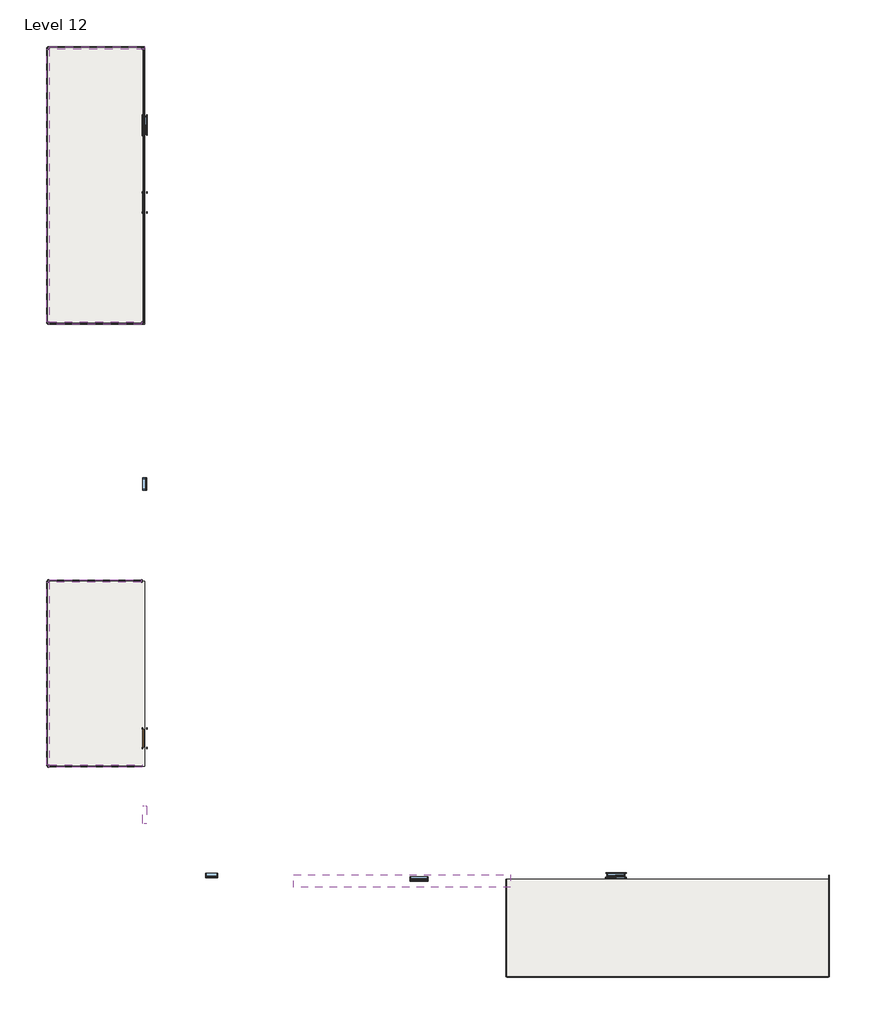
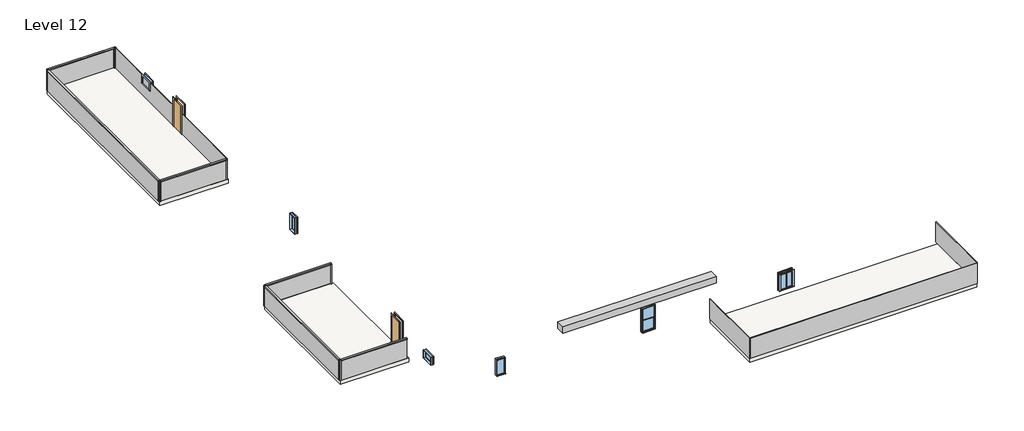
# One storey: 17 members, 10 plates, 6 windows, 3 slabs, 2 doors, 1 proxy.
"""IFC4 building model written with IfcOpenShell, lengths in millimetres."""

from ifc_helpers import new_model, si_unit, frame, origin, place, context, project, spatial, polyline, outline, extrude, transform, mapped, element, save
from components import generic_models_5_generic_models_5_6f0b94fe, door_54dd4da4, member_a0ba9e48, member_4491d118, member_6d14b308, member_9867d003, member_a33656d8, member_5f6c94d3, member_61d9bab4, system_panel_glazed_6303489a, system_panel_glazed_dbf8c7ac, system_panel_glazed_b7a52489, system_panel_glazed_1f759628, system_panel_glazed_82bc3a22, system_panel_glazed_e6d06af6, system_panel_glazed_929cc49f, system_panel_glazed_21f26c1a, system_panel_glazed_1fde7296, system_panel_glazed_b34c6f43, window_f274a882, window_80bd9af0, window_57c3ee1c, window_78885257, window_a4355bb3, window_54100e87

model = new_model("IFC4")

# Units and contexts
model_context = context("Model", 3, world=origin())
ifc_project = project(units=[si_unit("LENGTHUNIT", "METRE", prefix="MILLI")], contexts=[model_context])

# Site, building, storey
site = spatial("IfcSite", under=ifc_project)
building = spatial("IfcBuilding", under=site)
storey = spatial("IfcBuildingStorey", under=building, Name="Level 12", Elevation=19812.0)

# Proxy
placement = place(None, origin())
generic_models_5_generic_models_5_shape = generic_models_5_generic_models_5_6f0b94fe(model_context)
element("IfcBuildingElementProxy", 1, Name="Generic Models 5 : Generic Models 5", ObjectType="Generic Models 5 : Generic Models 5", at=placement, inside=storey, context=model_context, shape_type="MappedRepresentation", body=[
    mapped(generic_models_5_generic_models_5_shape, transform((508.0, 127.0, 0.0), x_axis=(1.0, 0.0, 0.0), y_axis=(0.0, 1.0, 0.0), z_axis=(0.0, 0.0, 1.0))),
])

# Doors
door_shape = door_54dd4da4(model_context)
element("IfcDoor", 2, ObjectType="Single-Flush : 36\" x 84\"", at=placement, inside=storey, context=model_context, shape_type="MappedRepresentation", body=[
    mapped(door_shape, transform((-15175.038074, 13037.8014639, 19812.0), x_axis=(0.0, 1.0, 0.0), y_axis=(-1.0, 0.0, 0.0), z_axis=(0.0, 0.0, 1.0))),
])
element("IfcDoor", 3, ObjectType="Single-Flush : 36\" x 84\"", at=placement, inside=storey, context=model_context, shape_type="MappedRepresentation", body=[
    mapped(door_shape, transform((-15175.038074, -13852.5915889, 19812.0), x_axis=(0.0, 1.0, 0.0), y_axis=(-1.0, 0.0, 0.0), z_axis=(0.0, 0.0, 1.0))),
])

# Members
member_shape = member_a0ba9e48(model_context)
element("IfcMember", 4, ObjectType="Rectangular Mullion : 2.5\" x 5\" rectangular", at=placement, inside=storey, context=model_context, shape_type="MappedRepresentation", body=[
    mapped(member_shape, transform((-15175.038074, 20810.2014639, 21336.0), x_axis=(0.0, 0.0, 1.0), y_axis=(0.0, -1.0, 0.0), z_axis=(1.0, 0.0, 0.0))),
])
member_2_shape = member_4491d118(model_context)
element("IfcMember", 5, ObjectType="Rectangular Mullion : 2.5\" x 5\" rectangular", at=placement, inside=storey, context=model_context, shape_type="MappedRepresentation", body=[
    mapped(member_2_shape, transform((-20051.838074, 20810.2014639, 19812.0), x_axis=(0.0, 1.0, 0.0), y_axis=(1.0, 0.0, 0.0), z_axis=(0.0, 0.0, -1.0))),
])
element("IfcMember", 6, ObjectType="Rectangular Mullion : 2.5\" x 5\" rectangular", at=placement, inside=storey, context=model_context, shape_type="MappedRepresentation", body=[
    mapped(member_2_shape, transform((-20051.838074, 6991.7543143, 19812.0), x_axis=(-1.0, 0.0, 0.0), y_axis=(0.0, 1.0, 0.0), z_axis=(0.0, 0.0, -1.0))),
])
element("IfcMember", 7, ObjectType="Rectangular Mullion : 2.5\" x 5\" rectangular", at=placement, inside=storey, context=model_context, shape_type="MappedRepresentation", body=[
    mapped(member_2_shape, transform((-15308.388074, -5966.8213044, 19812.0), x_axis=(1.0, 0.0, 0.0), y_axis=(0.0, -1.0, 0.0), z_axis=(0.0, 0.0, -1.0))),
])
element("IfcMember", 8, ObjectType="Rectangular Mullion : 2.5\" x 5\" rectangular", at=placement, inside=storey, context=model_context, shape_type="MappedRepresentation", body=[
    mapped(member_2_shape, transform((-20051.838074, -5966.8213044, 19812.0), x_axis=(0.0, 1.0, 0.0), y_axis=(1.0, 0.0, 0.0), z_axis=(0.0, 0.0, -1.0))),
])
element("IfcMember", 9, ObjectType="Rectangular Mullion : 2.5\" x 5\" rectangular", at=placement, inside=storey, context=model_context, shape_type="MappedRepresentation", body=[
    mapped(member_2_shape, transform((-20051.838074, -15250.5213044, 19812.0), x_axis=(-1.0, 0.0, 0.0), y_axis=(0.0, 1.0, 0.0), z_axis=(0.0, 0.0, -1.0))),
])
element("IfcMember", 10, ObjectType="Rectangular Mullion : 2.5\" x 5\" rectangular", at=placement, inside=storey, context=model_context, shape_type="MappedRepresentation", body=[
    mapped(member_2_shape, transform((-20051.838074, 20810.2014639, 21336.0), x_axis=(-1.0, 0.0, 0.0), y_axis=(0.0, -1.0, 0.0), z_axis=(0.0, 0.0, 1.0))),
])
element("IfcMember", 11, ObjectType="Rectangular Mullion : 2.5\" x 5\" rectangular", at=placement, inside=storey, context=model_context, shape_type="MappedRepresentation", body=[
    mapped(member_2_shape, transform((-20051.838074, 6991.7543143, 21336.0), x_axis=(0.0, -1.0, 0.0), y_axis=(1.0, 0.0, 0.0), z_axis=(0.0, 0.0, 1.0))),
])
element("IfcMember", 12, ObjectType="Rectangular Mullion : 2.5\" x 5\" rectangular", at=placement, inside=storey, context=model_context, shape_type="MappedRepresentation", body=[
    mapped(member_2_shape, transform((-15276.638074, 6991.7543143, 21336.0), x_axis=(1.0, 0.0, 0.0), y_axis=(0.0, 1.0, 0.0), z_axis=(0.0, 0.0, 1.0))),
])
element("IfcMember", 13, ObjectType="Rectangular Mullion : 2.5\" x 5\" rectangular", at=placement, inside=storey, context=model_context, shape_type="MappedRepresentation", body=[
    mapped(member_2_shape, transform((-20051.838074, -5966.8213044, 21336.0), x_axis=(-1.0, 0.0, 0.0), y_axis=(0.0, -1.0, 0.0), z_axis=(0.0, 0.0, 1.0))),
])
element("IfcMember", 14, ObjectType="Rectangular Mullion : 2.5\" x 5\" rectangular", at=placement, inside=storey, context=model_context, shape_type="MappedRepresentation", body=[
    mapped(member_2_shape, transform((-20051.838074, -15250.5213044, 21336.0), x_axis=(0.0, -1.0, 0.0), y_axis=(1.0, 0.0, 0.0), z_axis=(0.0, 0.0, 1.0))),
])
member_3_shape = member_6d14b308(model_context)
element("IfcMember", 15, ObjectType="Rectangular Mullion : 2.5\" x 5\" rectangular", at=placement, inside=storey, context=model_context, shape_type="MappedRepresentation", body=[
    mapped(member_3_shape, transform((-19988.338074, 6991.7543143, 21336.0), x_axis=(0.0, 0.0, 1.0), y_axis=(0.0, 1.0, 0.0), z_axis=(-1.0, 0.0, 0.0))),
])
element("IfcMember", 16, ObjectType="Rectangular Mullion : 2.5\" x 5\" rectangular", at=placement, inside=storey, context=model_context, shape_type="MappedRepresentation", body=[
    mapped(member_2_shape, transform((-15276.638074, 20810.2014639, 21336.0), x_axis=(0.0, 1.0, 0.0), y_axis=(-1.0, 0.0, 0.0), z_axis=(0.0, 0.0, 1.0))),
])
member_4_shape = member_9867d003(model_context)
element("IfcMember", 17, ObjectType="Rectangular Mullion : 2.5\" x 5\" rectangular", at=placement, inside=storey, context=model_context, shape_type="MappedRepresentation", body=[
    mapped(member_4_shape, transform((-20051.838074, 20746.7014639, 21336.0), x_axis=(0.0, 0.0, 1.0), y_axis=(1.0, 0.0, 0.0), z_axis=(0.0, 1.0, 0.0))),
])
member_5_shape = member_a33656d8(model_context)
element("IfcMember", 18, ObjectType="Rectangular Mullion : 2.5\" x 5\" rectangular", at=placement, inside=storey, context=model_context, shape_type="MappedRepresentation", body=[
    mapped(member_5_shape, transform((-15371.888074, -5966.8213044, 21336.0), x_axis=(0.0, 0.0, 1.0), y_axis=(0.0, -1.0, 0.0), z_axis=(1.0, 0.0, 0.0))),
])
member_6_shape = member_5f6c94d3(model_context)
element("IfcMember", 19, ObjectType="Rectangular Mullion : 2.5\" x 5\" rectangular", at=placement, inside=storey, context=model_context, shape_type="MappedRepresentation", body=[
    mapped(member_6_shape, transform((-20051.838074, -6030.3213044, 21336.0), x_axis=(0.0, 0.0, 1.0), y_axis=(1.0, 0.0, 0.0), z_axis=(0.0, 1.0, 0.0))),
])
member_7_shape = member_61d9bab4(model_context)
element("IfcMember", 20, ObjectType="Rectangular Mullion : 2.5\" x 5\" rectangular", at=placement, inside=storey, context=model_context, shape_type="MappedRepresentation", body=[
    mapped(member_7_shape, transform((-19988.338074, -15250.5213044, 21336.0), x_axis=(0.0, 0.0, 1.0), y_axis=(0.0, 1.0, 0.0), z_axis=(-1.0, 0.0, 0.0))),
])

# Plates
system_panel_glazed_shape = system_panel_glazed_6303489a(model_context)
element("IfcPlate", 21, ObjectType="System Panel : Glazed", at=placement, inside=storey, context=model_context, shape_type="MappedRepresentation", body=[
    mapped(system_panel_glazed_shape, transform((3011.361926, -23385.7985361, 19812.0), x_axis=(0.0, 1.0, 0.0), y_axis=(-1.0, 0.0, 0.0), z_axis=(0.0, 0.0, 1.0))),
])
system_panel_glazed_2_shape = system_panel_glazed_dbf8c7ac(model_context)
element("IfcPlate", 22, ObjectType="System Panel : Glazed", at=placement, inside=storey, context=model_context, shape_type="MappedRepresentation", body=[
    mapped(system_panel_glazed_2_shape, transform((11088.561926, -25824.1985361, 19812.0), x_axis=(-1.0, 0.0, 0.0), y_axis=(0.0, -1.0, 0.0), z_axis=(0.0, 0.0, 1.0))),
])
system_panel_glazed_3_shape = system_panel_glazed_b7a52489(model_context)
element("IfcPlate", 23, ObjectType="System Panel : Glazed", at=placement, inside=storey, context=model_context, shape_type="MappedRepresentation", body=[
    mapped(system_panel_glazed_3_shape, transform((19165.761926, -23284.1985361, 19812.0), x_axis=(0.0, -1.0, 0.0), y_axis=(1.0, 0.0, 0.0), z_axis=(0.0, 0.0, 1.0))),
])
system_panel_glazed_4_shape = system_panel_glazed_1f759628(model_context)
element("IfcPlate", 24, ObjectType="System Panel : Glazed", at=placement, inside=storey, context=model_context, shape_type="MappedRepresentation", body=[
    mapped(system_panel_glazed_4_shape, transform((-17664.238074, 6991.7543143, 19812.0), x_axis=(-1.0, 0.0, 0.0), y_axis=(0.0, -1.0, 0.0), z_axis=(0.0, 0.0, 1.0))),
])
system_panel_glazed_5_shape = system_panel_glazed_82bc3a22(model_context)
element("IfcPlate", 25, ObjectType="System Panel : Glazed", at=placement, inside=storey, context=model_context, shape_type="MappedRepresentation", body=[
    mapped(system_panel_glazed_5_shape, transform((-17581.688074, 20810.2014639, 19812.0), x_axis=(1.0, 0.0, 0.0), y_axis=(0.0, 1.0, 0.0), z_axis=(0.0, 0.0, 1.0))),
])
system_panel_glazed_6_shape = system_panel_glazed_e6d06af6(model_context)
element("IfcPlate", 26, ObjectType="System Panel : Glazed", at=placement, inside=storey, context=model_context, shape_type="MappedRepresentation", body=[
    mapped(system_panel_glazed_6_shape, transform((-15276.638074, 13869.2278891, 19812.0), x_axis=(0.0, -1.0, 0.0), y_axis=(1.0, 0.0, 0.0), z_axis=(0.0, 0.0, 1.0))),
])
system_panel_glazed_7_shape = system_panel_glazed_929cc49f(model_context)
element("IfcPlate", 27, ObjectType="System Panel : Glazed", at=placement, inside=storey, context=model_context, shape_type="MappedRepresentation", body=[
    mapped(system_panel_glazed_7_shape, transform((-20051.838074, 13900.9778891, 19812.0), x_axis=(0.0, 1.0, 0.0), y_axis=(-1.0, 0.0, 0.0), z_axis=(0.0, 0.0, 1.0))),
])
system_panel_glazed_8_shape = system_panel_glazed_21f26c1a(model_context)
element("IfcPlate", 28, ObjectType="System Panel : Glazed", at=placement, inside=storey, context=model_context, shape_type="MappedRepresentation", body=[
    mapped(system_panel_glazed_8_shape, transform((-17680.113074, -5966.8213044, 19812.0), x_axis=(1.0, 0.0, 0.0), y_axis=(0.0, 1.0, 0.0), z_axis=(0.0, 0.0, 1.0))),
])
system_panel_glazed_9_shape = system_panel_glazed_1fde7296(model_context)
element("IfcPlate", 29, ObjectType="System Panel : Glazed", at=placement, inside=storey, context=model_context, shape_type="MappedRepresentation", body=[
    mapped(system_panel_glazed_9_shape, transform((-20051.838074, -10608.6713044, 19812.0), x_axis=(0.0, 1.0, 0.0), y_axis=(-1.0, 0.0, 0.0), z_axis=(0.0, 0.0, 1.0))),
])
system_panel_glazed_10_shape = system_panel_glazed_b34c6f43(model_context)
element("IfcPlate", 30, ObjectType="System Panel : Glazed", at=placement, inside=storey, context=model_context, shape_type="MappedRepresentation", body=[
    mapped(system_panel_glazed_10_shape, transform((-17648.363074, -15250.5213044, 19812.0), x_axis=(-1.0, 0.0, 0.0), y_axis=(0.0, -1.0, 0.0), z_axis=(0.0, 0.0, 1.0))),
])

# Slabs
element("IfcSlab", 31, ObjectType="Generic - 12\"", at=placement, inside=storey, context=model_context, shape_type="SweptSolid", body=[
    extrude(outline(polyline([(3011.361926, -20947.3985361), (19165.761926, -20947.3985361), (19165.761926, -25824.1985361), (3011.361926, -25824.1985361), (3011.361926, -20947.3985361)])), frame((0.0, 0.0, 19507.2), z_axis=(0.0, 0.0, 1.0), x_axis=(1.0, 0.0, 0.0)), (0.0, 0.0, 1.0), 304.8),
])
element("IfcSlab", 32, ObjectType="Generic - 12\"", at=placement, inside=storey, context=model_context, shape_type="SweptSolid", body=[
    extrude(outline(polyline([(-20051.838074, -15263.2213044), (-20051.838074, -5966.8213044), (-15175.038074, -5966.8213044), (-15175.038074, -15263.2213044), (-20051.838074, -15263.2213044)])), frame((0.0, 0.0, 19507.2), z_axis=(0.0, 0.0, 1.0), x_axis=(1.0, 0.0, 0.0)), (0.0, 0.0, 1.0), 304.8),
])
element("IfcSlab", 33, ObjectType="Generic - 12\"", at=placement, inside=storey, context=model_context, shape_type="SweptSolid", body=[
    extrude(outline(polyline([(-20051.838074, 20810.2014639), (-15175.038074, 20810.2014639), (-15175.038074, 6941.8014639), (-20051.838074, 6941.8014639), (-20051.838074, 20810.2014639)])), frame((0.0, 0.0, 19507.2), z_axis=(0.0, 0.0, 1.0), x_axis=(1.0, 0.0, 0.0)), (0.0, 0.0, 1.0), 304.8),
])

# Windows
window_shape = window_f274a882(model_context)
element("IfcWindow", 34, ObjectType="Double Hung : 36\" x 72\"", at=placement, inside=storey, context=model_context, shape_type="MappedRepresentation", body=[
    mapped(window_shape, transform((-1408.238074, -20921.9985361, 20192.5798521), x_axis=(-1.0, 0.0, 0.0), y_axis=(0.0, -1.0, 0.0), z_axis=(0.0, 0.0, 1.0))),
])
window_2_shape = window_80bd9af0(model_context)
element("IfcWindow", 35, ObjectType="Fixed : 24\" x 48\"", at=placement, inside=storey, context=model_context, shape_type="MappedRepresentation", body=[
    mapped(window_2_shape, transform((-15175.038074, -1128.1213044, 19812.0), x_axis=(0.0, -1.0, 0.0), y_axis=(1.0, 0.0, 0.0), z_axis=(0.0, 0.0, 1.0))),
])
window_3_shape = window_57c3ee1c(model_context)
element("IfcWindow", 36, ObjectType="Fixed : 36\" x 24\"", at=placement, inside=storey, context=model_context, shape_type="MappedRepresentation", body=[
    mapped(window_3_shape, transform((-15175.038074, -17739.7213044, 20102.4980928), x_axis=(0.0, -1.0, 0.0), y_axis=(1.0, 0.0, 0.0), z_axis=(0.0, 0.0, 1.0))),
])
window_4_shape = window_78885257(model_context)
element("IfcWindow", 37, ObjectType="Instance - Fixed : 24\" x 48\"", at=placement, inside=storey, context=model_context, shape_type="MappedRepresentation", body=[
    mapped(window_4_shape, transform((-11860.338074, -20744.1985361, 19812.0), x_axis=(-1.0, 0.0, 0.0), y_axis=(0.0, -1.0, 0.0), z_axis=(0.0, 0.0, 1.0))),
])
window_5_shape = window_a4355bb3(model_context)
element("IfcWindow", 38, ObjectType="Slider with Trim : 36\" x 24\"", at=placement, inside=storey, context=model_context, shape_type="MappedRepresentation", body=[
    mapped(window_5_shape, transform((-15175.038074, 16924.0014639, 19812.0), x_axis=(0.0, 1.0, 0.0), y_axis=(-1.0, 0.0, 0.0), z_axis=(0.0, 0.0, 1.0))),
])
window_6_shape = window_54100e87(model_context)
element("IfcWindow", 39, ObjectType="Slider with Trim : 36\" x 48\"", at=placement, inside=storey, context=model_context, shape_type="MappedRepresentation", body=[
    mapped(window_6_shape, transform((8497.761926, -20744.1985361, 19179.6342809), x_axis=(-1.0, 0.0, 0.0), y_axis=(0.0, -1.0, 0.0), z_axis=(0.0, 0.0, 1.0))),
])

save(model, "model.ifc")

# Revit data of these elements
# Type "Single-Flush : 36\" x 84\""
#   Type Mark = "1"
#   Construction Type Id = "MDOOR"
#   Assembly Code = "C1020"
#   Analytic Construction = "Metal"
#   Thickness = 0' - 2"
#   Heat Transfer Coefficient (U) = 0.651978 BTU/(h·ft²·°F)
#   Height = 7' - 0"
#   Trim Projection Ext = 0' - 1"
#   Trim Projection Int = 0' - 1"
#   Trim Width = 0' - 3"
#   Width = 3' - 0"
#   Define Thermal Properties by = 1
#   Door Material = Door - Panel
#   Frame Material = Door - Frame
#   Visual Light Transmittance = 0
#   Solar Heat Gain Coefficient = 0
#   Function = (empty or 0)
#   Wall Closure = (empty or 0)
# Type "Rectangular Mullion : 2.5\" x 5\" rectangular"
#   built-in parameter 1007304 = 0.416667 (stored number, unit not read)
#   built-in parameter 1007301 = 0.104167 (stored number, unit not read)
#   built-in parameter 1007300 = 0.104167 (stored number, unit not read)
# Type "System Panel : Glazed"
#   Construction Type Id = "GSP4R"
#   Analytic Construction = "1/8 in Pilkington single glazing"
#   Visual Light Transmittance = 0.9
#   Solar Heat Gain Coefficient = 0.86
#   Heat Transfer Coefficient (U) = 1.18115 BTU/(h·ft²·°F)
# Type "Generic - 12\""
#   Assembly Code = "B1010"
#   Function = 0
#   Layers, outside or top first: 1' - 0" no material (function 1)
# Type "Double Hung : 36\" x 72\""
#   Type Mark = "18"
#   Construction Type Id = "GSP4R"
#   Assembly Code = "B2020100"
#   Analytic Construction = "1/8 in Pilkington single glazing"
#   Visual Light Transmittance = 0.9
#   Solar Heat Gain Coefficient = 0.78
#   Heat Transfer Coefficient (U) = 0.6496 BTU/(h·ft²·°F)
#   Height = 6' - 0"
#   Default Sill Height = 1' - 0"
#   Width = 3' - 0"
#   Window Inset = 0' - 0 3/4"
#   Define Thermal Properties by = 1
#   Glass Pane Material = Glass
#   Sash Material = Sash
#   Description = (empty or 0)
#   Wall Closure = (empty or 0)
# Type "Fixed : 24\" x 48\""
#   Type Mark = "2"
#   Construction Type Id = "GSP4R"
#   Assembly Code = "B2020100"
#   Analytic Construction = "1/8 in Pilkington single glazing"
#   Visual Light Transmittance = 0.9
#   Solar Heat Gain Coefficient = 0.78
#   Heat Transfer Coefficient (U) = 0.6496 BTU/(h·ft²·°F)
#   Height = 4' - 0"
#   Default Sill Height = 3' - 0"
#   Width = 2' - 0"
#   Window Inset = 0' - 0 3/4"
#   Define Thermal Properties by = 1
#   Glass Pane Material = Glass
#   Sash Material = Sash
#   Wall Closure = (empty or 0)
# Type "Fixed : 36\" x 24\""
#   Type Mark = "8"
#   Construction Type Id = "GSP4R"
#   Assembly Code = "B2020100"
#   Analytic Construction = "1/8 in Pilkington single glazing"
#   Visual Light Transmittance = 0.9
#   Solar Heat Gain Coefficient = 0.78
#   Heat Transfer Coefficient (U) = 0.6496 BTU/(h·ft²·°F)
#   Height = 2' - 0"
#   Default Sill Height = 3' - 0"
#   Width = 3' - 0"
#   Window Inset = 0' - 0 3/4"
#   Define Thermal Properties by = 1
#   Glass Pane Material = Glass
#   Sash Material = Sash
#   Wall Closure = (empty or 0)
# Type "Instance - Fixed : 24\" x 48\""
#   Type Mark = "19"
#   Construction Type Id = "GSP4R"
#   Assembly Code = "B2020100"
#   Analytic Construction = "1/8 in Pilkington single glazing"
#   Visual Light Transmittance = 0.9
#   Thermal Resistance (R) = 0.8466 (h·ft²·°F)/BTU
#   Solar Heat Gain Coefficient = 0.86
#   Heat Transfer Coefficient (U) = 1.1812 BTU/(h·ft²·°F)
#   Height [instance default] = 4' - 0"
#   Default Sill Height = 3' - 0"
#   Width [instance default] = 2' - 0"
#   Window Inset = 0' - 0 3/4"
#   Define Thermal Properties by = 1
#   Glass Pane Material = Glass
#   Sash Material = Sash
#   Wall Closure = (empty or 0)
# Type "Slider with Trim : 36\" x 24\""
#   Type Mark = "23"
#   Construction Type Id = "GSP4R"
#   Assembly Code = "B2020100"
#   Analytic Construction = "1/8 in Pilkington single glazing"
#   Visual Light Transmittance = 0.9
#   Solar Heat Gain Coefficient = 0.78
#   Heat Transfer Coefficient (U) = 0.6496 BTU/(h·ft²·°F)
#   Height = 2' - 0"
#   Default Sill Height = 3' - 0"
#   Trim Projection - Ext. = 0' - 0 3/4"
#   Trim Projection - Int. = 0' - 0 3/4"
#   Trim Width - Exterior = 0' - 3 1/2"
#   Trim Width - Interior = 0' - 3 1/2"
#   Width = 3' - 0"
#   Window Inset = 0' - 0 3/4"
#   Define Thermal Properties by = 1
#   Glass Pane Material = Glass
#   Sash Material = Sash
#   Trim Exterior Material = Trim
#   Trim Interior Material = Trim
#   Wall Closure = (empty or 0)
# Type "Slider with Trim : 36\" x 48\""
#   Type Mark = "22"
#   Construction Type Id = "GSP4R"
#   Assembly Code = "B2020100"
#   Analytic Construction = "1/8 in Pilkington single glazing"
#   Visual Light Transmittance = 0.9
#   Solar Heat Gain Coefficient = 0.78
#   Heat Transfer Coefficient (U) = 0.6496 BTU/(h·ft²·°F)
#   Height = 4' - 0"
#   Default Sill Height = 3' - 0"
#   Trim Projection - Ext. = 0' - 0 3/4"
#   Trim Projection - Int. = 0' - 0 3/4"
#   Trim Width - Exterior = 0' - 3 1/2"
#   Trim Width - Interior = 0' - 3 1/2"
#   Width = 3' - 0"
#   Window Inset = 0' - 0 3/4"
#   Define Thermal Properties by = 1
#   Glass Pane Material = Glass
#   Sash Material = Sash
#   Trim Exterior Material = Trim
#   Trim Interior Material = Trim
#   Wall Closure = (empty or 0)
# Element 1 (IfcBuildingElementProxy, "Generic Models 5 : Generic Models 5")
#   Phase Created = New Construction
# Elements 2, 3 (IfcDoor, "Single-Flush : 36\" x 84\"")
#   Phase Created = New Construction
#   Materials on its faces: "Door - Frame", "Door - Panel"
# Elements 4, 5, 6, 7, 8, 9, 10, 11, 12, 13, 14, 15, 16, 17, 18, 19, 20 (IfcMember, "Rectangular Mullion : 2.5\" x 5\" rectangular")
#   Phase Created = New Construction
#   Materials on its faces: "Aluminum"
# Elements 21, 22, 23, 24, 25, 26, 27, 28, 29, 30 (IfcPlate, "System Panel : Glazed")
#   Phase Created = New Construction
#   Materials on its faces: "Glass"
# Elements 31, 32, 33 (IfcSlab, "Generic - 12\"")
#   built-in parameter 1001955 = 3.14159 (stored number, unit not read)
#   Height Offset From Level = 0' - 0"
#   Phase Created = New Construction
#   Materials on its faces: "Default Floor"
# Element 34 (IfcWindow, "Double Hung : 36\" x 72\"")
#   Mark = "6"
#   Phase Created = New Construction
#   Materials on its faces: "Sash", "Glass"
# Element 35 (IfcWindow, "Fixed : 24\" x 48\"")
#   Mark = "50"
#   Phase Created = New Construction
#   Materials on its faces: "Sash", "Glass"
# Element 36 (IfcWindow, "Fixed : 36\" x 24\"")
#   Mark = "72"
#   Phase Created = New Construction
#   Materials on its faces: "Sash", "Glass"
# Element 37 (IfcWindow, "Instance - Fixed : 24\" x 48\"")
#   Mark = "16"
#   Width = 2' - 0"
#   Height = 4' - 0"
#   Phase Created = New Construction
#   Materials on its faces: "Sash", "Glass"
# Element 38 (IfcWindow, "Slider with Trim : 36\" x 24\"")
#   Mark = "61"
#   Phase Created = New Construction
#   Materials on its faces: "Sash", "Trim", "Glass"
# Element 39 (IfcWindow, "Slider with Trim : 36\" x 48\"")
#   Mark = "28"
#   Phase Created = New Construction
#   Materials on its faces: "Sash", "Trim", "Glass"
# Materials
#   "Door - Panel": class "Wood", colour RGB 210 159 95, transparency 0
#   "Door - Frame": colour RGB 118 70 51, transparency 0
#   "Glass": class "Glass", colour RGB 0 128 192, transparency 0.75, Description = "Soda Lime Glass", Cost = 0
#   "Sash": class "Wood", colour RGB 224 178 126, transparency 0
#   "Trim": class "Wood", colour RGB 224 178 126, transparency 0
#   "Aluminum": class "Metal", colour RGB 247 247 247, transparency 0, Description = "Aluminum 6061", Cost = 0
#   "Default Floor": colour RGB 128 128 128, transparency 0
